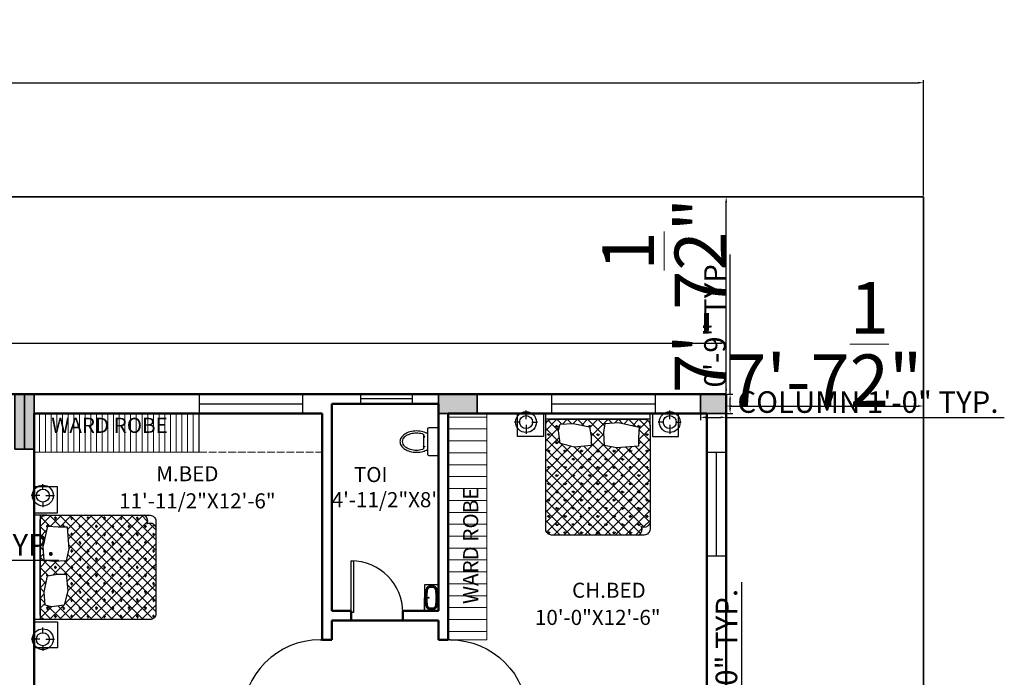
# Model space of a CAD drawing. Units: inches. Extents: x 2214 to 3937, y 762 to 2085.
# Tile 9 of 9: x 3243 to 3700, y 1780 to 2085. Entities that reach past the tile are written whole.
import ezdxf

# ---------------------------------------------------------------- set-up
doc = ezdxf.new("R2010")
doc.units = ezdxf.units.IN
doc.linetypes.add('ACAD_ISO02W100', pattern=[15, 12, -3])
for name, color, linetype, lineweight in [('A-ANNO-DIMS', 2, 'Continuous', 18), ('A-ANNO-TEXT', 7, 'Continuous', 18), ('A-AREA-IDEN', 7, 'Continuous', 25), ('A-CASE-OVHD', 252, 'ACAD_ISO02W100', 13), ('A-CASE-PATT', 252, 'Continuous', 13), ('A-COLS', 5, 'Continuous', 35), ('A-FLOR-FIXT', 9, 'Continuous', 18), ('A-FURN', 8, 'Continuous', 18), ('C-ANNO-DIMS', 2, 'Continuous', 18), ('C-PROP', 3, 'Continuous', 35), ('door', 122, 'Continuous', 25), ('wall', 20, 'Continuous', 50), ('wardrobe', 252, 'Continuous', 18), ('window', 4, 'Continuous', 25)]:
    doc.layers.add(name, color=color, linetype=linetype, lineweight=lineweight)
for name, color, linetype in [('GIUONG', 70, 'Continuous'), ('NOI THAT', 42, 'Continuous'), ('THIET-BI', 21, 'Continuous')]:
    doc.layers.add(name, color=color, linetype=linetype)
doc.styles.get("Standard").update_dxf_attribs({"font": 'arial.ttf'})
doc.dimstyles.new('ISO-25', dxfattribs={"dimtxt": 10, "dimasz": 2.5, "dimexe": 1.25, "dimexo": 0.625, "dimtad": 1, "dimdec": 1, "dimlunit": 4, "dimtxsty": 'Standard', "dimcen": 2.5, "dimadec": 0, "dimazin": 0, "dimtfac": 1, "dimtdec": 1, "dimtmove": 0, "dimatfit": 3, "dimfxl": 1, "dimarcsym": 0})

# ---------------------------------------------------------------- blocks, each defined once
blk = doc.blocks.new('*U2')
for p, q in [((0, 0), (0, -6)), ((40, 0), (40, -6))]:
    blk.add_line(p, q)
blk.add_lwpolyline([(0, 0), (0, 40), (1.75, 40), (1.75, 0)], close=True)
blk.add_arc((0, 0), 40, 0, 90)
blk = doc.blocks.new('*X8')
at = {"color": 0}
for p, q in [((0, 0), (0, 0)), ((-707, -141), (-734, -115)), ((-707, -141), (-707, -104)), ((-707, -141), (-681, -115)), ((-566, 0), (-566, 0)), ((-566, 0), (-566, 0)), ((-283, 0), (-283, 0)), ((-283, 0), (-283, 0)), ((-156, -126), (-168, -115)), ((-141, -141), (-142, -140)), ((-141, -141), (-141, -104)), ((-141, -141), (-115, -115)), ((120, -120), (115, -115)), ((283, 0), (283, 0)), ((566, 0), (566, 0)), ((699, -134), (681, -115)), ((707, -135), (707, -104)), ((710, -139), (734, -115)), ((-849, -283), (-875, -256)), ((-849, -283), (-849, -245)), ((-849, -283), (-822, -256)), ((0, -283), (-27, -256)), ((0, -283), (0, -245)), ((0, -283), (27, -256)), ((849, -283), (822, -256)), ((849, -283), (849, -245)), ((849, -283), (875, -256)), ((-707, -424), (-734, -398)), ((-707, -424), (-707, -387)), ((-707, -424), (-681, -398)), ((-116, -399), (-115, -398)), ((707, -424), (703, -420)), ((707, -424), (707, -387)), ((707, -424), (734, -398)), ((-849, -566), (-875, -539)), ((-849, -566), (-849, -528)), ((-849, -566), (-822, -539)), ((-707, -707), (-707, -670)), ((-566, -566), (-592, -539)), ((-566, -566), (-566, -528)), ((-566, -566), (-539, -539)), ((-424, -707), (-424, -670)), ((-283, -566), (-309, -539)), ((-283, -566), (-283, -528)), ((-283, -566), (-256, -539)), ((-141, -707), (-141, -670)), ((0, -566), (-27, -539)), ((0, -566), (0, -528)), ((0, -566), (27, -539)), ((141, -707), (141, -670)), ((283, -566), (256, -539)), ((283, -566), (283, -528)), ((283, -566), (309, -539)), ((424, -707), (424, -670)), ((566, -566), (539, -539)), ((566, -566), (566, -528)), ((566, -566), (592, -539)), ((707, -707), (707, -670)), ((849, -566), (822, -539)), ((849, -566), (849, -528)), ((849, -566), (875, -539)), ((-849, -849), (-875, -822)), ((-849, -849), (-849, -811)), ((-849, -849), (-822, -822)), ((-707, -707), (-734, -681)), ((-707, -707), (-681, -681)), ((-566, -849), (-592, -822)), ((-566, -849), (-566, -811)), ((-566, -849), (-539, -822)), ((-424, -707), (-451, -681)), ((-424, -707), (-398, -681)), ((-283, -849), (-309, -822)), ((-283, -849), (-283, -811)), ((-283, -849), (-256, -822)), ((-141, -707), (-168, -681)), ((-141, -707), (-115, -681)), ((0, -849), (-27, -822)), ((0, -849), (0, -811)), ((0, -849), (27, -822)), ((141, -707), (115, -681)), ((141, -707), (168, -681)), ((283, -849), (256, -822)), ((283, -849), (283, -811)), ((283, -849), (309, -822)), ((424, -707), (398, -681)), ((424, -707), (451, -681)), ((566, -849), (539, -822)), ((566, -849), (566, -811)), ((566, -849), (592, -822)), ((707, -707), (681, -681)), ((707, -707), (734, -681)), ((849, -849), (822, -822)), ((849, -849), (849, -811)), ((849, -849), (875, -822)), ((-707, -990), (-734, -963)), ((-707, -990), (-707, -952)), ((-707, -990), (-681, -963)), ((-424, -990), (-451, -963)), ((-424, -990), (-424, -952)), ((-424, -990), (-398, -963)), ((-141, -990), (-168, -963)), ((-141, -990), (-141, -952)), ((-141, -990), (-115, -963)), ((141, -990), (115, -963)), ((141, -990), (141, -952)), ((141, -990), (168, -963)), ((424, -990), (398, -963)), ((424, -990), (424, -952)), ((424, -990), (451, -963)), ((707, -990), (681, -963)), ((707, -990), (707, -952)), ((707, -990), (734, -963)), ((-849, -1131), (-875, -1105)), ((-849, -1131), (-849, -1094)), ((-849, -1131), (-822, -1105)), ((-566, -1131), (-592, -1105)), ((-566, -1131), (-566, -1094)), ((-566, -1131), (-539, -1105)), ((-283, -1131), (-309, -1105)), ((-283, -1131), (-283, -1094)), ((-283, -1131), (-256, -1105)), ((0, -1131), (-27, -1105)), ((0, -1131), (0, -1094)), ((0, -1131), (27, -1105)), ((283, -1131), (256, -1105)), ((283, -1131), (283, -1094)), ((283, -1131), (309, -1105)), ((566, -1131), (539, -1105)), ((566, -1131), (566, -1094)), ((566, -1131), (592, -1105)), ((849, -1131), (822, -1105)), ((849, -1131), (849, -1094)), ((849, -1131), (875, -1105)), ((-707, -1273), (-734, -1246)), ((-707, -1273), (-707, -1235)), ((-707, -1273), (-681, -1246)), ((-424, -1273), (-451, -1246)), ((-424, -1273), (-424, -1235)), ((-424, -1273), (-398, -1246)), ((-141, -1273), (-168, -1246)), ((-141, -1273), (-141, -1235)), ((-141, -1273), (-115, -1246)), ((141, -1273), (115, -1246)), ((141, -1273), (141, -1235)), ((141, -1273), (168, -1246)), ((424, -1273), (398, -1246)), ((424, -1273), (424, -1235)), ((424, -1273), (451, -1246)), ((707, -1273), (681, -1246)), ((707, -1273), (707, -1235)), ((707, -1273), (734, -1246)), ((-849, -1414), (-875, -1388)), ((-849, -1414), (-849, -1377)), ((-849, -1414), (-822, -1388)), ((-707, -1556), (-734, -1529)), ((-707, -1556), (-707, -1518)), ((-707, -1556), (-681, -1529)), ((-566, -1414), (-592, -1388)), ((-566, -1414), (-566, -1377)), ((-566, -1414), (-539, -1388)), ((-424, -1556), (-451, -1529)), ((-424, -1556), (-424, -1518)), ((-424, -1556), (-398, -1529)), ((-283, -1414), (-309, -1388)), ((-283, -1414), (-283, -1377)), ((-283, -1414), (-256, -1388)), ((-141, -1556), (-168, -1529)), ((-141, -1556), (-141, -1518)), ((-141, -1556), (-115, -1529)), ((0, -1414), (-27, -1388)), ((0, -1414), (0, -1377)), ((0, -1414), (27, -1388)), ((141, -1556), (115, -1529)), ((141, -1556), (141, -1518)), ((141, -1556), (168, -1529)), ((283, -1414), (256, -1388)), ((283, -1414), (283, -1377)), ((283, -1414), (309, -1388)), ((424, -1556), (398, -1529)), ((424, -1556), (424, -1518)), ((424, -1556), (451, -1529)), ((566, -1414), (539, -1388)), ((566, -1414), (566, -1377)), ((566, -1414), (592, -1388)), ((707, -1556), (681, -1529)), ((707, -1556), (707, -1518)), ((707, -1556), (734, -1529)), ((849, -1414), (822, -1388)), ((849, -1414), (849, -1377)), ((849, -1414), (875, -1388)), ((-849, -1697), (-875, -1671)), ((-849, -1697), (-849, -1660)), ((-849, -1697), (-822, -1671)), ((-566, -1697), (-592, -1671)), ((-566, -1697), (-566, -1660)), ((-566, -1697), (-539, -1671)), ((-283, -1697), (-309, -1671)), ((-283, -1697), (-283, -1660)), ((-283, -1697), (-256, -1671)), ((0, -1697), (-27, -1671)), ((0, -1697), (0, -1660)), ((0, -1697), (27, -1671)), ((283, -1697), (256, -1671)), ((283, -1697), (283, -1660)), ((283, -1697), (309, -1671)), ((566, -1697), (539, -1671)), ((566, -1697), (566, -1660)), ((566, -1697), (592, -1671)), ((849, -1697), (822, -1671)), ((849, -1697), (849, -1660)), ((849, -1697), (875, -1671)), ((-707, -1838), (-734, -1812)), ((-707, -1838), (-707, -1801)), ((-707, -1838), (-681, -1812)), ((-424, -1838), (-451, -1812)), ((-424, -1838), (-424, -1801)), ((-424, -1838), (-398, -1812)), ((-141, -1838), (-168, -1812)), ((-141, -1838), (-141, -1801)), ((-141, -1838), (-115, -1812)), ((141, -1838), (115, -1812)), ((141, -1838), (141, -1801)), ((141, -1838), (168, -1812)), ((424, -1838), (398, -1812)), ((424, -1838), (424, -1801)), ((424, -1838), (451, -1812)), ((707, -1838), (681, -1812)), ((707, -1838), (707, -1801)), ((707, -1838), (734, -1812)), ((-849, -1980), (-875, -1953)), ((-849, -1980), (-849, -1942)), ((-849, -1980), (-822, -1953)), ((-566, -1980), (-592, -1953)), ((-566, -1980), (-566, -1942)), ((-566, -1980), (-539, -1953)), ((-283, -1980), (-309, -1953)), ((-283, -1980), (-283, -1942)), ((-283, -1980), (-256, -1953)), ((0, -1980), (-27, -1953)), ((0, -1980), (0, -1942)), ((0, -1980), (27, -1953)), ((283, -1980), (256, -1953)), ((283, -1980), (283, -1942)), ((283, -1980), (309, -1953)), ((566, -1980), (539, -1953)), ((566, -1980), (566, -1942)), ((566, -1980), (592, -1953))]:
    blk.add_line(p, q, dxfattribs=at)
blk = doc.blocks.new('*X7')
at = {"color": 0}
for p, q in [((-900, -193), (-707, 0)), ((-623, -84), (-707, 0)), ((-614, -83), (-530, 0)), ((-457, -74), (-530, 0)), ((-425, -72), (-354, 0)), ((-245, -108), (-354, 0)), ((-278, -101), (-177, 0)), ((103, -280), (-177, 0)), ((-142, -142), (0, 0)), ((-117, -294), (177, 0)), ((120, -120), (0, 0)), ((241, -64), (177, 0)), ((292, -61), (354, 0)), ((426, -72), (354, 0)), ((452, -78), (530, 0)), ((654, -123), (530, 0)), ((596, -111), (707, 0)), ((900, -193), (707, 0)), ((-900, -370), (-667, -137)), ((-656, -405), (-900, -161)), ((-683, -201), (-862, -22)), ((703, -358), (900, -161)), ((708, -175), (862, -22)), ((-900, -1254), (101, -252)), ((-900, -546), (-668, -314)), ((735, -1973), (-900, -337)), ((-763, -2000), (900, -337)), ((900, -1254), (-128, -225)), ((900, -370), (708, -178)), ((-900, -1430), (112, -418)), ((-900, -723), (-605, -429)), ((-900, -900), (-465, -465)), ((-900, -1077), (-293, -470)), ((-900, -1607), (231, -476)), ((-900, -1784), (394, -489)), ((-888, -1948), (586, -475)), ((801, -1862), (-641, -419)), ((900, -1784), (-404, -480)), ((900, -1607), (-243, -465)), ((900, -1430), (-116, -415)), ((900, -1077), (317, -494)), ((900, -900), (483, -483)), ((900, -723), (647, -470)), ((900, -546), (703, -349)), ((586, -2000), (-900, -514)), ((-586, -2000), (900, -514)), ((409, -2000), (-900, -691)), ((-409, -2000), (900, -691)), ((232, -2000), (-900, -868)), ((-232, -2000), (900, -868)), ((55, -2000), (-900, -1045)), ((-55, -2000), (900, -1045)), ((-121, -2000), (-900, -1221)), ((121, -2000), (900, -1221)), ((-298, -2000), (-900, -1398)), ((298, -2000), (900, -1398)), ((-475, -2000), (-900, -1575)), ((475, -2000), (900, -1575)), ((-652, -2000), (-900, -1752)), ((790, -1861), (900, -1752)), ((-835, -1994), (-894, -1935)), ((652, -2000), (761, -1890))]:
    blk.add_line(p, q, dxfattribs=at)
blk = doc.blocks.new('A$C190D2546')
at = {"layer": 'GIUONG'}
for points in [[(787, 1584), (758, 1799), (787, 1914), (1016, 1928), (1296, 1871), (1325, 1699), (1325, 1548), (1038, 1519)], [(1555, 1548), (1541, 1771), (1569, 1928), (1799, 1943), (2151, 1864), (2144, 1685), (2144, 1534), (1763, 1505)]]:
    blk.add_lwpolyline(points, close=True, dxfattribs=at)
for centre, radius in [((200, 1951), 180), ((200, 1951), 112), ((2682, 1951), 180), ((2682, 1951), 112)]:
    blk.add_circle(centre, radius, dxfattribs=at)
at = {"layer": 'NOI THAT'}
for p, q in [((200, 2001), (200, 2151)), ((541, 2100), (2341, 2100)), ((541, 1881), (541, 2100)), ((2341, 1881), (2341, 2100)), ((2682, 2001), (2682, 2151)), ((100, 1951), (0, 1951)), ((200, 1901), (200, 1751)), ((300, 1951), (400, 1951)), ((2341, 2000), (541, 2000)), ((2582, 1951), (2482, 1951)), ((2682, 1901), (2682, 1751)), ((2782, 1951), (2882, 1951))]:
    blk.add_line(p, q, dxfattribs=at)
for points in [[(500, 2101), (500, 1701), (50, 1701), (50, 2101)], [(2382, 2101), (2382, 1701), (2832, 1701), (2832, 2101)]]:
    blk.add_lwpolyline(points, close=True, dxfattribs=at)
blk.add_lwpolyline([(641, 2000), (2241, 2000, -0.414214), (2341, 1900), (2341, 100, -0.414214), (2241, 0), (641, 0, -0.414214), (541, 100), (541, 1900, -0.414214)], format="xyb", close=True, dxfattribs=at)
for centre, start, end in [((2241, 250), 243.4349, 333.4349), ((2091, 100), 296.5651, 26.5651)]:
    blk.add_arc(centre, 112, start, end, dxfattribs=at)
for name in ['*X7', '*X8']:
    blk.add_blockref(name, (1441, 2000), dxfattribs=at)
blk = doc.blocks.new('A$C65B13726')
at = {"layer": 'THIET-BI'}
for p, q in [((0, 400), (0, 200)), ((0, 400), (375, 400)), ((134, 362), (621, 360)), ((375, 291), (357, 291)), ((357, 291), (393, 291)), ((375, 291), (375, 309)), ((375, 309), (375, 274)), ((134, 39), (616, 39))]:
    blk.add_line(p, q, dxfattribs=at)
blk.add_lwpolyline([(0, 400), (0, 0), (750, 0), (750, 400)], close=True, dxfattribs=at)
blk.add_lwpolyline([(714, 200), (714, 240, 0.341607), (621, 360), (598, 366, 0.001439), (593, 367, 0.035276), (375, 382, 0.035276), (157, 367, 0.001439), (152, 366), (129, 360, 0.341607), (36, 240), (36, 200), (36, 161, 0.341607), (129, 40), (152, 34, 0.001439), (157, 33, 0.035276), (375, 18, 0.035276), (593, 33, 0.001439), (598, 34), (621, 40, 0.341607), (714, 161)], format="xyb", close=True, dxfattribs=at)
for points in [[(323, 348, 0.026733), (162, 334, 0.000876), (159, 333), (137, 327, 0.341782), (70, 240), (70, 161, 0.341782), (137, 73), (159, 67, 0.000876), (162, 67, 0.026747), (323, 52, 0.035276)], [(337, 337, 0.028876), (163, 323, 0.00069), (161, 322), (140, 317, 0.341861), (81, 240), (81, 160, 0.341861), (140, 83), (161, 78, 0.00069), (163, 77, 0.028898), (337, 63, 0.035276)], [(407, 348, 0.00526), (375, 349, 0.005313), (343, 348, 0.000876)], [(394, 338, 0.003179), (375, 338, 0.003179), (356, 338, 0.00069)], [(375, 382), (375, 382, 0.025118)], [(375, 382), (375, 382, 0.035276)], [(669, 200), (669, 240, 0.341861), (610, 317), (589, 322, 0.00069), (587, 323, 0.028876), (413, 337, 0.003179)], [(680, 200), (680, 240, 0.341782), (613, 327), (591, 333, 0.000876), (588, 334, 0.026733), (427, 348, 0.006503)], [(343, 52, 0.005316), (375, 52, 0.005263), (407, 52, 0.000876)], [(356, 62, 0.003135), (375, 62, 0.003135), (394, 62, 0.00069)], [(375, 17), (375, 17, 0.035276)], [(413, 63, 0.028961), (587, 77, 0.00069), (589, 78), (610, 83, 0.341861), (669, 160), (669, 200)], [(427, 52, 0.026747), (588, 67, 0.000876), (591, 67), (613, 73, 0.341782), (680, 161), (680, 200)]]:
    blk.add_lwpolyline(points, format="xyb", dxfattribs=at)
blk.add_circle((375, 291), 14.5, dxfattribs=at)
for centre, radius, start, end in [((375, 400), 73.6, 211.9576, 327.7237), ((324, 352), 19.1, 310.8832, 28.9258), ((375, 400), 65.2, 239.0852, 300.5961), ((426, 351), 19.1, 150.7555, 228.798), ((375, 0), 73.6, 32.2763, 148.0424), ((324, 48), 19.1, 331.0742, 49.1168), ((375, 0), 65.2, 59.4039, 120.9148), ((426, 49), 19.1, 131.202, 209.2445)]:
    blk.add_arc(centre, radius, start, end, dxfattribs=at)
blk = doc.blocks.new('A$C5AF77858')
at = {"layer": 'THIET-BI'}
for p, q in [((0, 675), (0, 525)), ((475, 700), (25, 700)), ((500, 525), (500, 675)), ((25, 500), (475, 500)), ((117, 430), (383, 430)), ((154, 452), (154, 430)), ((164, 452), (154, 452)), ((154, 430), (164, 430)), ((164, 430), (164, 452)), ((336, 430), (336, 452)), ((336, 452), (346, 452)), ((346, 430), (336, 430)), ((346, 452), (346, 430))]:
    blk.add_line(p, q, dxfattribs=at)
for centre, radius, start, end in [((25, 675), 25, 90, 180), ((475, 675), 25, 0, 90), ((25, 525), 25, 180, 270), ((514, 299), 458, 164.9269, 180), ((384, 334), 323, 149.0966, 164.9269), ((514, 299), 418, 164.9269, 180), ((384, 334), 283, 160.176, 164.9269), ((116, 334), 283, 15.0731, 19.824), ((-14, 299), 418, 0, 15.0731), ((116, 334), 323, 15.0731, 30.9034), ((-14, 299), 458, 0, 15.0731), ((475, 525), 25, 270, 0), ((514, 299), 458, 180, 195.0731), ((384, 264), 323, 195.0731, 213.0315), ((514, 299), 418, 180, 195.0731), ((384, 264), 283, 195.0731, 213.0315), ((116, 264), 283, 326.9685, 344.9269), ((116, 264), 323, 326.9685, 344.9269), ((-14, 299), 418, 344.9269, 0), ((-14, 299), 458, 344.9269, 0), ((302, 210), 226, 213.0315, 237.5002), ((302, 210), 186, 213.0315, 237.5002), ((250, 129), 129, 237.5002, 270), ((250, 129), 89.3, 237.5002, 270), ((250, 129), 89.3, 270, 302.4998), ((250, 129), 129, 270, 302.4998), ((198, 210), 186, 302.4998, 326.9685), ((198, 210), 226, 302.4998, 326.9685)]:
    blk.add_arc(centre, radius, start, end, dxfattribs=at)
blk = doc.blocks.new('*D19')
at = {"layer": 'C-ANNO-DIMS', "color": 0, "lineweight": -2, "ltscale": 0.3, "transparency": 16777216}
for p, q in [((2582.56, 2003.84), (2582.56, 2057.46)), ((2585.06, 2056.21), (3660.06, 2056.21)), ((3662.56, 2003.84), (3662.56, 2057.46))]:
    blk.add_line(p, q, dxfattribs=at)
at = {"layer": 'C-ANNO-DIMS', "color": 0, "ltscale": 0.3, "transparency": 16777216}
for points in [[(2585.06, 2056.63), (2585.06, 2055.8), (2582.56, 2056.21)], [(3660.06, 2056.63), (3660.06, 2055.8), (3662.56, 2056.21)]]:
    blk.add_solid(points, dxfattribs=at)
at = {"layer": 'Defpoints', "color": 0, "ltscale": 0.3, "transparency": 16777216}
for p in [(3662.56, 2056.21), (2582.56, 2003.22), (3662.56, 2003.22)]:
    blk.add_point(p, dxfattribs=at)
at = {"layer": 'C-ANNO-DIMS', "color": 0, "ltscale": 0.3, "transparency": 16777216, "insert": (3122.56, 2069.09), "char_height": 24, "attachment_point": 5}
blk.add_mtext("90'", dxfattribs=at)
blk = doc.blocks.new('*D21')
at = {"layer": 'C-ANNO-DIMS', "color": 0, "lineweight": -2, "ltscale": 0.3, "transparency": 16777216}
for p, q in [((3571.06, 1911.09), (3571.06, 1904.93)), ((3662.56, 1911.09), (3662.56, 1904.93)), ((3573.56, 1906.18), (3660.06, 1906.18))]:
    blk.add_line(p, q, dxfattribs=at)
at = {"layer": 'C-ANNO-DIMS', "color": 0, "ltscale": 0.3, "transparency": 16777216}
for points in [[(3573.56, 1906.6), (3573.56, 1905.77), (3571.06, 1906.18)], [(3660.06, 1906.6), (3660.06, 1905.77), (3662.56, 1906.18)]]:
    blk.add_solid(points, dxfattribs=at)
at = {"layer": 'Defpoints', "color": 0, "ltscale": 0.3, "transparency": 16777216}
for p in [(3571.06, 1911.72), (3662.56, 1911.72), (3662.56, 1906.18)]:
    blk.add_point(p, dxfattribs=at)
at = {"layer": 'C-ANNO-DIMS', "color": 0, "ltscale": 0.3, "transparency": 16777216, "insert": (3616.81, 1934.91), "char_height": 24, "attachment_point": 5}
blk.add_mtext('7\'-7{\\H1x;\\S1/2;}"', dxfattribs=at)
blk = doc.blocks.new('*D22')
at = {"layer": 'C-ANNO-DIMS', "color": 0, "lineweight": -2, "ltscale": 0.3, "transparency": 16777216}
for p, q in [((3571.06, 1914.22), (3571.06, 2000.72)), ((3571.68, 2003.22), (3572.31, 2003.22)), ((3571.68, 1911.72), (3572.31, 1911.72))]:
    blk.add_line(p, q, dxfattribs=at)
at = {"layer": 'C-ANNO-DIMS', "color": 0, "ltscale": 0.3, "transparency": 16777216}
for points in [[(3570.64, 2000.72), (3571.47, 2000.72), (3571.06, 2003.22)], [(3570.64, 1914.22), (3571.47, 1914.22), (3571.06, 1911.72)]]:
    blk.add_solid(points, dxfattribs=at)
at = {"layer": 'Defpoints', "color": 0, "ltscale": 0.3, "transparency": 16777216}
for p in [(3571.06, 2003.22), (3571.06, 2003.22), (3571.06, 1911.72)]:
    blk.add_point(p, dxfattribs=at)
at = {"layer": 'C-ANNO-DIMS', "color": 0, "ltscale": 0.3, "transparency": 16777216, "insert": (3542.33, 1957.47), "char_height": 24, "attachment_point": 5, "rotation": 90}
blk.add_mtext('7\'-7{\\H1x;\\S1/2;}"', dxfattribs=at)
blk = doc.blocks.new('*D25')
at = {"layer": 'A-ANNO-DIMS', "color": 0, "lineweight": -2, "ltscale": 0.3, "transparency": 16777216}
for p, q in [((2674.06, 1912.34), (2674.06, 1936.65)), ((2676.56, 1935.4), (3568.56, 1935.4)), ((3571.06, 1912.34), (3571.06, 1936.65))]:
    blk.add_line(p, q, dxfattribs=at)
at = {"layer": 'A-ANNO-DIMS', "color": 0, "ltscale": 0.3, "transparency": 16777216}
for points in [[(2676.56, 1935.82), (2676.56, 1934.98), (2674.06, 1935.4)], [(3568.56, 1935.82), (3568.56, 1934.98), (3571.06, 1935.4)]]:
    blk.add_solid(points, dxfattribs=at)
at = {"layer": 'Defpoints', "color": 0, "ltscale": 0.3, "transparency": 16777216}
for p in [(3571.06, 1935.4), (2674.06, 1911.72), (3571.06, 1911.72)]:
    blk.add_point(p, dxfattribs=at)
at = {"layer": 'A-ANNO-DIMS', "color": 0, "ltscale": 0.3, "transparency": 16777216, "insert": (3122.56, 1948.28), "char_height": 24, "attachment_point": 5}
blk.add_mtext('74\'-9"', dxfattribs=at)
blk = doc.blocks.new('COL-25_5X9')
at = {"ltscale": 0.3}
h = blk.add_hatch(color=256, dxfattribs=at)
h.dxf.hatch_style = 1
h.paths.add_polyline_path([(25.5, 0), (25.5, 9), (0, 9), (0, 0)])
for p, q in [((25.5, 9), (25.5, 0)), ((0, 4.5), (25.5, 4.5)), ((0, 4.5), (0, 0)), ((0, 0), (4.5, 0))]:
    blk.add_line(p, q)
blk.add_lwpolyline([(0, 9), (25.5, 9), (25.5, 0), (0, 0)], close=True, dxfattribs=at)
blk = doc.blocks.new('COL-18X9')
at = {"ltscale": 0.3}
h = blk.add_hatch(color=256, dxfattribs=at)
h.dxf.hatch_style = 1
h.paths.add_polyline_path([(18, 0), (18, 9), (0, 9), (0, 0)])
blk.add_lwpolyline([(0, 9), (18, 9), (18, 0), (0, 0)], close=True, dxfattribs=at)
blk = doc.blocks.new('COL-12X9')
at = {"ltscale": 0.3}
h = blk.add_hatch(color=256, dxfattribs=at)
h.dxf.hatch_style = 1
h.paths.add_polyline_path([(12, 0), (12, 9), (0, 9), (0, 0)])
blk.add_lwpolyline([(12, 0), (0, 0), (0, 9), (12, 9)], close=True, dxfattribs=at)
blk = doc.blocks.new('WIN-48X9')
for p, q in [((0, 48), (9, 48)), ((0, 0), (9, 0))]:
    blk.add_line(p, q)
at = {"ltscale": 0.3}
blk.add_line((4.5, 0), (4.5, 48), dxfattribs=at)
blk = doc.blocks.new('WIN-24X4_5')
for p, q in [((0, 0), (0, 4.5)), ((24, 0), (24, 4.5))]:
    blk.add_line(p, q)
at = {"ltscale": 0.3}
blk.add_line((24, 2.25), (0, 2.25), dxfattribs=at)
blk = doc.blocks.new('*D39')
at = {"layer": 'C-ANNO-DIMS', "color": 0, "lineweight": -2, "ltscale": 0.3, "transparency": 16777216}
for p, q in [((3559.06, 1902.09), (3559.06, 1899.67)), ((3561.56, 1900.92), (3568.56, 1900.92)), ((3571.06, 1902.09), (3571.06, 1899.67)), ((3571.06, 1900.92), (3700.07, 1900.92))]:
    blk.add_line(p, q, dxfattribs=at)
at = {"layer": 'C-ANNO-DIMS', "color": 0, "ltscale": 0.3, "transparency": 16777216}
for points in [[(3561.56, 1901.34), (3561.56, 1900.5), (3559.06, 1900.92)], [(3568.56, 1901.34), (3568.56, 1900.5), (3571.06, 1900.92)]]:
    blk.add_solid(points, dxfattribs=at)
at = {"layer": 'Defpoints', "color": 0, "ltscale": 0.3, "transparency": 16777216}
for p in [(3559.06, 1902.72), (3571.06, 1902.72), (3571.06, 1900.92)]:
    blk.add_point(p, dxfattribs=at)
at = {"layer": 'C-ANNO-DIMS', "color": 0, "ltscale": 0.3, "transparency": 16777216, "insert": (3636.81, 1906.72), "char_height": 10, "attachment_point": 5}
blk.add_mtext('COLUMN 1\'-0" TYP.', dxfattribs=at)
blk = doc.blocks.new('*D40')
at = {"layer": 'C-ANNO-DIMS', "color": 0, "lineweight": -2, "ltscale": 0.3, "transparency": 16777216}
for p, q in [((3572.86, 1911.72), (3572.86, 1976.42)), ((3571.68, 1911.72), (3574.11, 1911.72)), ((3572.86, 1905.22), (3572.86, 1909.22)), ((3571.68, 1902.72), (3574.11, 1902.72))]:
    blk.add_line(p, q, dxfattribs=at)
at = {"layer": 'C-ANNO-DIMS', "color": 0, "ltscale": 0.3, "transparency": 16777216}
for points in [[(3572.44, 1909.22), (3573.27, 1909.22), (3572.86, 1911.72)], [(3572.44, 1905.22), (3573.27, 1905.22), (3572.86, 1902.72)]]:
    blk.add_solid(points, dxfattribs=at)
at = {"layer": 'Defpoints', "color": 0, "ltscale": 0.3, "transparency": 16777216}
for p in [(3571.06, 1911.72), (3572.86, 1911.72), (3571.06, 1902.72)]:
    blk.add_point(p, dxfattribs=at)
at = {"layer": 'C-ANNO-DIMS', "color": 0, "ltscale": 0.3, "transparency": 16777216, "insert": (3567.13, 1945.32), "char_height": 10, "attachment_point": 5, "rotation": 90}
blk.add_mtext('0\'-9" TYP.', dxfattribs=at)
blk = doc.blocks.new('*D41')
at = {"layer": 'C-ANNO-DIMS', "color": 0, "lineweight": -2, "ltscale": 0.3, "transparency": 16777216}
for p, q in [((3578.26, 1694.22), (3578.26, 1824.51)), ((3571.68, 1694.22), (3579.51, 1694.22)), ((3578.26, 1648.72), (3578.26, 1691.72)), ((3571.68, 1646.22), (3579.51, 1646.22))]:
    blk.add_line(p, q, dxfattribs=at)
at = {"layer": 'C-ANNO-DIMS', "color": 0, "ltscale": 0.3, "transparency": 16777216}
for points in [[(3577.84, 1691.72), (3578.67, 1691.72), (3578.26, 1694.22)], [(3577.84, 1648.72), (3578.67, 1648.72), (3578.26, 1646.22)]]:
    blk.add_solid(points, dxfattribs=at)
at = {"layer": 'Defpoints', "color": 0, "ltscale": 0.3, "transparency": 16777216}
for p in [(3571.06, 1694.22), (3578.26, 1694.22), (3571.06, 1646.22)]:
    blk.add_point(p, dxfattribs=at)
at = {"layer": 'C-ANNO-DIMS', "color": 0, "ltscale": 0.3, "transparency": 16777216, "insert": (3572.46, 1760.61), "char_height": 10, "attachment_point": 5, "rotation": 90}
blk.add_mtext('WINDOW 4\'-0" TYP.', dxfattribs=at)
blk = doc.blocks.new('*D45')
at = {"layer": 'C-ANNO-DIMS', "color": 0, "lineweight": -2, "ltscale": 0.3, "transparency": 16777216}
for p, q in [((3063.9, 1845.7), (3063.9, 1833.47)), ((3141.29, 1845.7), (3141.29, 1833.47)), ((3066.4, 1834.72), (3138.79, 1834.72)), ((3141.29, 1834.72), (3261.46, 1834.72))]:
    blk.add_line(p, q, dxfattribs=at)
at = {"layer": 'C-ANNO-DIMS', "color": 0, "ltscale": 0.3, "transparency": 16777216}
for points in [[(3066.4, 1835.13), (3066.4, 1834.3), (3063.9, 1834.72)], [(3138.79, 1835.13), (3138.79, 1834.3), (3141.29, 1834.72)]]:
    blk.add_solid(points, dxfattribs=at)
at = {"layer": 'Defpoints', "color": 0, "ltscale": 0.3, "transparency": 16777216}
for p in [(3063.9, 1846.33), (3141.29, 1846.33), (3141.29, 1834.72)]:
    blk.add_point(p, dxfattribs=at)
at = {"layer": 'C-ANNO-DIMS', "color": 0, "ltscale": 0.3, "transparency": 16777216, "insert": (3202.62, 1840.51), "char_height": 10, "attachment_point": 5}
blk.add_mtext('BED 6\'-5 1/2" TYP.', dxfattribs=at)

msp = doc.modelspace()

# ---------------------------------------------------------------- hatches: boundary and pattern name
at = {"layer": 'A-CASE-PATT', "ltscale": 0.3}
h = msp.add_hatch(dxfattribs=at)
h.set_pattern_fill('ANSI31', color=256, scale=0.830844, angle=45, style=0)
h.paths.add_polyline_path([(3250.06, 1884.72), (3326.56, 1884.72), (3326.56, 1902.72), (3250.06, 1902.72)])
h = msp.add_hatch(dxfattribs=at)
h.set_pattern_fill('ANSI31', color=256, scale=1.74057, angle=-45, style=0)
h.paths.add_polyline_path([(3442.06, 1797.72), (3460.06, 1797.72), (3460.06, 1902.72), (3442.06, 1902.72)])

# ---------------------------------------------------------------- linework, layer by layer
at = {"layer": 'A-CASE-OVHD', "ltscale": 0.3}
msp.add_line((3326.56, 1884.72), (3383.56, 1884.72), dxfattribs=at)
at = {"layer": 'C-PROP'}
for p, q in [((2582.56, 2003.22), (3662.56, 2003.22)), ((3662.56, 2003.22), (3662.56, 1355.22))]:
    msp.add_line(p, q, dxfattribs=at)
at = {"layer": 'wall'}
for p, q in [((2674.06, 1911.72), (3571.06, 1911.72)), ((3571.06, 1911.72), (3571.06, 1475.22)), ((3388.06, 1907.22), (3437.56, 1907.22)), ((3388.06, 1811.22), (3388.06, 1907.22)), ((3437.56, 1811.22), (3437.56, 1907.22)), ((3250.06, 1902.72), (3383.56, 1902.72)), ((3250.06, 1752.72), (3250.06, 1902.72)), ((3383.56, 1797.72), (3383.56, 1902.72)), ((3442.06, 1902.72), (3562.06, 1902.72)), ((3442.06, 1797.72), (3442.06, 1902.72)), ((3562.06, 1902.72), (3562.06, 1752.72)), ((3388.06, 1811.22), (3397.06, 1811.22)), ((3397.06, 1811.22), (3397.06, 1806.72)), ((3421.06, 1811.22), (3421.06, 1806.72)), ((3421.06, 1811.22), (3437.56, 1811.22)), ((3388.06, 1806.72), (3437.56, 1806.72)), ((3388.06, 1797.72), (3388.06, 1806.72)), ((3437.56, 1797.72), (3437.56, 1806.72)), ((3383.56, 1797.72), (3388.06, 1797.72)), ((3442.06, 1797.72), (3437.56, 1797.72))]:
    msp.add_line(p, q, dxfattribs=at)
at = {"layer": 'wardrobe'}
for p, q in [((3326.56, 1884.72), (3326.56, 1902.72)), ((3326.56, 1902.72), (3326.56, 1884.72)), ((3460.06, 1797.72), (3460.06, 1902.72)), ((3250.06, 1884.72), (3326.56, 1884.72)), ((3442.06, 1797.72), (3460.06, 1797.72))]:
    msp.add_line(p, q, dxfattribs=at)

# ---------------------------------------------------------------- block references
at = {"layer": 'A-COLS', "rotation": 269.9999999999964}
msp.add_blockref('COL-25_5X9', (3241.06, 1911.72), dxfattribs=at)
at = {"layer": 'A-COLS'}
for name, p in [('COL-18X9', (3437.56, 1902.73)), ('COL-12X9', (3559.06, 1902.72))]:
    msp.add_blockref(name, p, dxfattribs=at)
at = {"layer": 'A-FLOR-FIXT'}
for name, p, xscale, yscale, zscale, rotation in [('A$C5AF77858', (3419.73, 1896.03), 0.0254713121376822, 0.0254713121376822, 0.0254713121376822, 270), ('A$C65B13726', (3437.56, 1811.22), 0.0160009442456078, 0.0160009442456078, 0.0160009442456078, 89.99999999999999)]:
    msp.add_blockref(name, p, dxfattribs=dict(at, xscale=xscale, yscale=yscale, zscale=zscale, rotation=rotation))
at = {"layer": 'A-FURN', "xscale": 0.0268541596481872, "yscale": 0.0268541596481872, "zscale": 0.0268541596481872}
msp.add_blockref('A$C190D2546', (3472.84, 1846.33), dxfattribs=at)
at = {"layer": 'A-FURN', "xscale": 0.0268541596481872, "yscale": 0.0268541596481872, "zscale": 0.0268541596481872, "rotation": 90}
msp.add_blockref('A$C190D2546', (3306.45, 1792.6), dxfattribs=at)
at = {"layer": 'door', "xscale": 0.6000000000000114, "yscale": 0.6000000000000114, "zscale": 0.6000000000000114}
msp.add_blockref('*U2', (3397.06, 1810.32), dxfattribs=at)
at = {"layer": 'door', "yscale": 0.9, "zscale": 0.9}
for p, xscale, rotation in [((3382.66, 1761.72), 0.9, 90), ((3442.96, 1761.72), -0.9, 270)]:
    msp.add_blockref('*U2', p, dxfattribs=dict(at, xscale=xscale, rotation=rotation))
at = {"layer": 'window'}
for p, rotation in [((3326.56, 1911.72), 270.0000000000023), ((3490.06, 1911.72), 270.0000000000017)]:
    msp.add_blockref('WIN-48X9', p, dxfattribs=dict(at, rotation=rotation))
for name, p in [('WIN-24X4_5', (3401.56, 1907.22)), ('WIN-48X9', (3562.06, 1836.72))]:
    msp.add_blockref(name, p, dxfattribs=at)

# ---------------------------------------------------------------- texts
at = {"layer": 'A-ANNO-TEXT', "ltscale": 0.3}
msp.add_text('WARD ROBE', height=7, dxfattribs=at).set_placement((3257.97, 1893.72))
msp.add_text('WARD ROBE', height=7, rotation=90, dxfattribs=at).set_placement((3456.01, 1814.3))
at = {"layer": 'A-AREA-IDEN', "ltscale": 0.3}
for s, p in [('M.BED', (3306.64, 1871.27)), ('TOI', (3398.35, 1870.88)), ('11\'-11/2"X12\'-6"', (3289.42, 1858.67)), ('4\'-11/2"X8\'', (3388.06, 1859.22)), ('CH.BED', (3499.55, 1817.2)), ('10\'-0"X12\'-6"', (3482.34, 1804.6))]:
    msp.add_text(s, height=7, dxfattribs=at).set_placement(p)

# ---------------------------------------------------------------- dimensions: what is measured, and where the dimension line sits
at = {"layer": 'A-ANNO-DIMS', "ltscale": 0.3}
dim = msp.add_linear_dim(base=(3571.06, 1935.4), p1=(2674.06, 1911.72), p2=(3571.06, 1911.72), dimstyle='ISO-25', override={"dimtxt": 24, "dimclrd": 0, "dimclre": 0, "dimclrt": 0}, dxfattribs=at)
dim.commit()
dim.dimension.update_dxf_attribs({"geometry": '*D25', "text_midpoint": (3122.56, 1948.28)})
at = {"layer": 'C-ANNO-DIMS', "ltscale": 0.3}
for base, p1, p2, picture, middle in [((3662.56, 2056.21), (2582.56, 2003.22), (3662.56, 2003.22), '*D19', (3122.56, 2069.09)), ((3662.56, 1906.18), (3571.06, 1911.72), (3662.56, 1911.72), '*D21', (3616.81, 1934.91))]:
    dim = msp.add_linear_dim(base=base, p1=p1, p2=p2, dimstyle='ISO-25', override={"dimtxt": 24, "dimclrd": 0, "dimclre": 0, "dimclrt": 0}, dxfattribs=at)
    dim.commit()
    dim.dimension.update_dxf_attribs({"geometry": picture, "text_midpoint": middle})
dim = msp.add_linear_dim(base=(3571.06, 2003.22), p1=(3571.06, 1911.72), p2=(3571.06, 2003.22), angle=90, dimstyle='ISO-25', override={"dimtxt": 24, "dimclrd": 0, "dimclre": 0, "dimclrt": 0}, dxfattribs=at)
dim.commit()
dim.dimension.update_dxf_attribs({"geometry": '*D22', "text_midpoint": (3542.33, 1957.47)})
for base, p1, p2, text, picture, middle in [((3572.86, 1911.72), (3571.06, 1902.72), (3571.06, 1911.72), '<> TYP.', '*D40', (3567.13, 1945.32)), ((3578.26, 1694.22), (3571.06, 1646.22), (3571.06, 1694.22), 'WINDOW <> TYP.', '*D41', (3572.46, 1760.61))]:
    dim = msp.add_linear_dim(base=base, p1=p1, p2=p2, angle=90, text=text, dimstyle='ISO-25', override={"dimdec": 1, "dimlfac": 1, "dimrnd": 0, "dimzin": 1, "dimdsep": 46, "dimlunit": 4, "dimfrac": 2}, dxfattribs=at)
    dim.commit()
    dim.dimension.update_dxf_attribs({"geometry": picture, "text_midpoint": middle})
for base, p1, p2, text, picture, middle in [((3571.06, 1900.92), (3559.06, 1902.72), (3571.06, 1902.72), 'COLUMN <> TYP.', '*D39', (3636.81, 1906.72)), ((3141.29, 1834.72), (3063.9, 1846.33), (3141.29, 1846.33), 'BED <> TYP.', '*D45', (3202.62, 1840.51))]:
    dim = msp.add_linear_dim(base=base, p1=p1, p2=p2, text=text, dimstyle='ISO-25', override={"dimdec": 1, "dimlfac": 1, "dimrnd": 0, "dimzin": 1, "dimdsep": 46, "dimlunit": 4, "dimfrac": 2}, dxfattribs=at)
    dim.commit()
    dim.dimension.update_dxf_attribs({"geometry": picture, "text_midpoint": middle})

doc.saveas('drawing.dxf')
